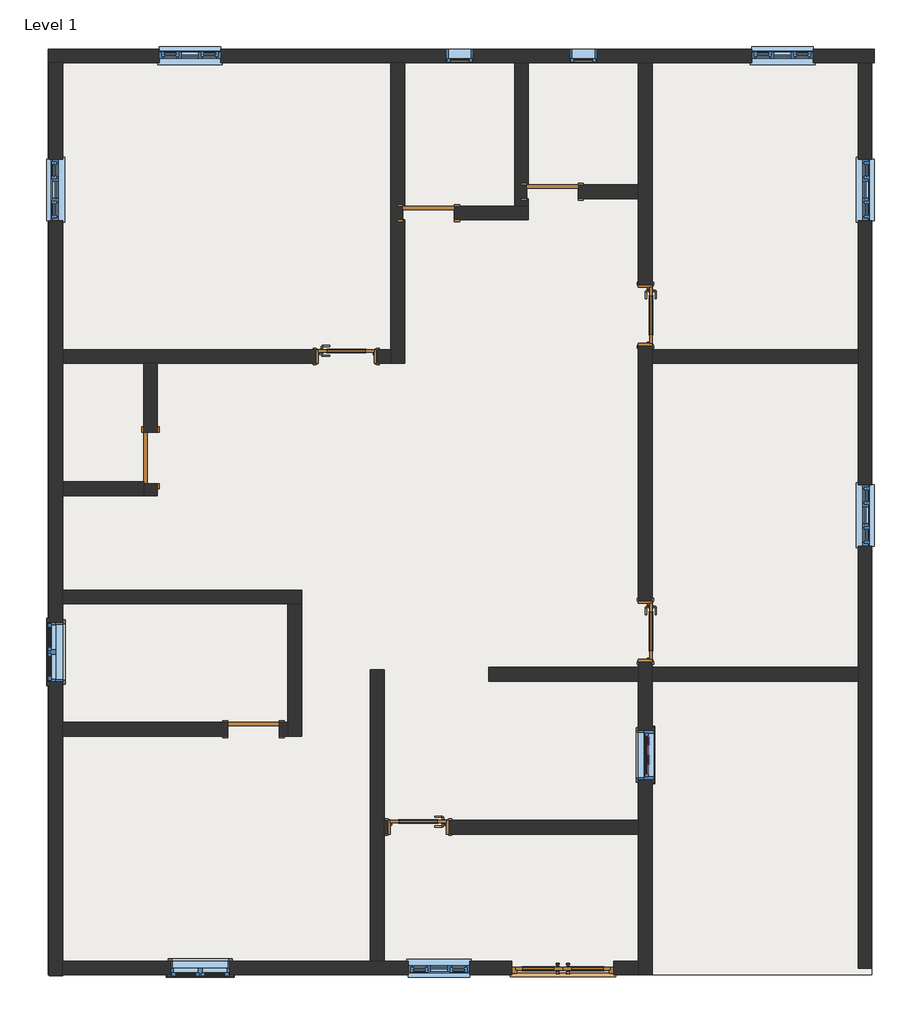
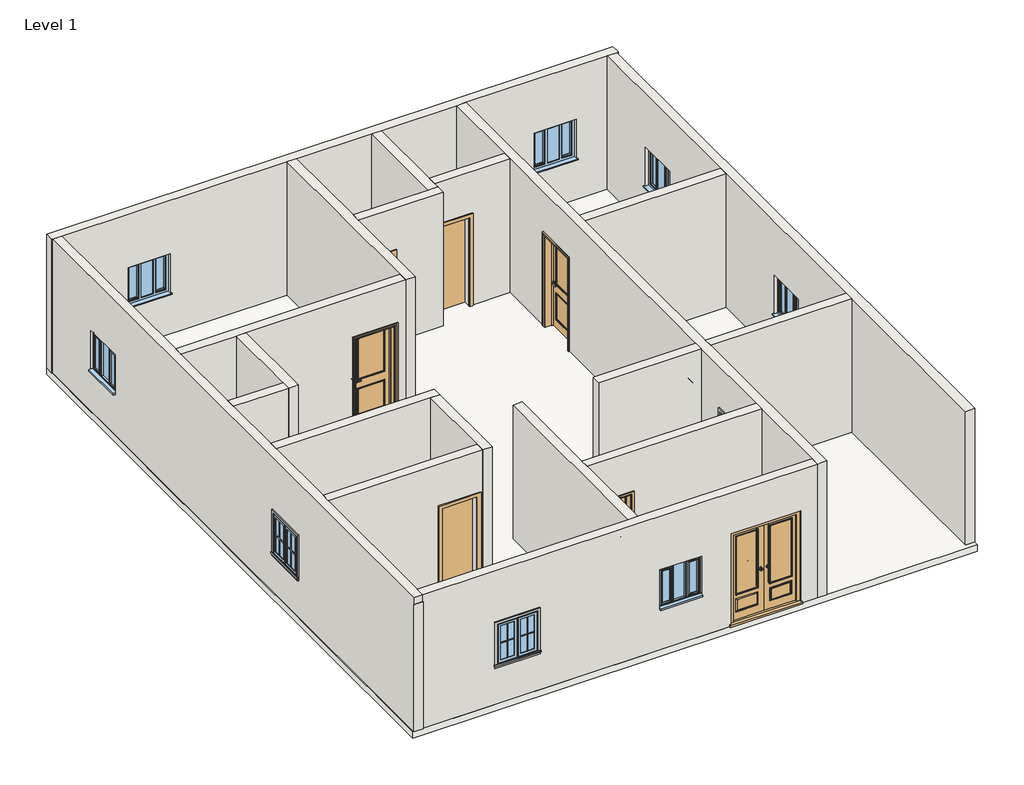
# One storey, incomplete: 19 walls, 12 proxies, 11 windows, 9 doors, 1 slab.
# Revit data of these elements (continued)
# Element 43 (IfcWindow, "Fixed : 16\" x 24\"") (continued)
#   Materials on its faces: "Sash", "Glass"
# Element 44 (IfcWindow, "Window-Casement-Double : 34\" x 36\"")
#   Mark = "1"
#   Window Inset = 0' - 0"
#   Interior Wall Closure = 0' - 2 1/4"
#   Frame Extension = 0' - 0 1/4"
#   Exterior Wall Closure = 0' - 1 1/4"
#   Interior Trim Visibility = yes
#   Exterior Trim Visibility = yes
#   Phase Created = New Construction
#   Materials on its faces: "Wood - Stained", "Glass", "Clad - White"
# Element 45 (IfcWindow, "Window-Casement-Double : 34\" x 36\"")
#   Mark = "2"
#   Window Inset = 0' - 0"
#   Interior Wall Closure = 0' - 2 1/4"
#   Frame Extension = 0' - 0 1/4"
#   Exterior Wall Closure = 0' - 1 1/4"
#   Interior Trim Visibility = yes
#   Exterior Trim Visibility = yes
#   Phase Created = New Construction
#   Materials on its faces: "Wood - Stained", "Glass", "Clad - White"
# Element 46 (IfcWindow, "Window-Double-Hung : 28\" x 46\"")
#   Mark = "11"
#   Window Inset = 0' - 0"
#   Interior Wall Closure = 0' - 1 1/2"
#   Frame Extension = 0' - 1 1/4"
#   Exterior Wall Closure = 0' - 0 1/2"
#   Interior Trim Visibility = yes
#   Indicator Visibility = yes
#   Exterior Trim Visibility = yes
#   Phase Created = New Construction
#   Materials on its faces: "Wood - Stained", "Glass", "Clad - White"
# Element 47 (IfcWindow, "Windows_Tpl_Plain : 910x910mm")
#   Mark = "3"
#   Phase Created = New Construction
#   Materials on its faces: "Window Frame", "Glass"
# Element 48 (IfcWindow, "Windows_Tpl_Plain : 910x910mm")
#   Mark = "6"
#   Phase Created = New Construction
#   Materials on its faces: "Window Frame", "Glass"
# Element 49 (IfcWindow, "Windows_Tpl_Plain : 910x910mm")
#   Mark = "7"
#   Phase Created = New Construction
#   Materials on its faces: "Window Frame", "Glass"
# Element 50 (IfcWindow, "Windows_Tpl_Plain : 910x910mm")
#   Mark = "8"
#   Phase Created = New Construction
#   Materials on its faces: "Window Frame", "Glass"
# Element 51 (IfcWindow, "Windows_Tpl_Plain : 910x910mm")
#   Mark = "4"
#   Phase Created = New Construction
#   Materials on its faces: "Window Frame", "Glass"
# Element 52 (IfcWindow, "Windows_Tpl_Plain : 910x910mm")
#   Mark = "5"
#   Phase Created = New Construction
#   Materials on its faces: "Window Frame", "Glass"
# Materials
#   "Door - Panel": class "Wood", colour RGB 210 159 95, transparency 0, Cost = 0
#   "Door - Glazing": colour RGB 0 0 255, transparency 0.75
#   "Door - Frame/Mullion": class "Wood", colour RGB 212 179 113, transparency 0
#   "Door - Handle": colour RGB 247 247 247, transparency 0
#   "Door - Architrave": class "Wood", colour RGB 154 90 5, transparency 0
#   "Door - Frame": colour RGB 118 70 51, transparency 0, Cost = 0
#   "Glass": class "Glass", colour RGB 0 128 192, transparency 0.75, Description = "Soda Lime Glass", Cost = 0
#   "Sash": class "Wood", colour RGB 224 178 126, transparency 0, Cost = 0
#   "Wood - Stained": class "Wood", colour RGB 224 178 126, transparency 0, Cost = 0
#   "Clad - White": class "Wood", colour RGB 242 242 238, transparency 0, Cost = 0
#   "Window Frame": colour RGB 249 249 249, transparency 0
#   "Default Floor": colour RGB 128 128 128, transparency 0, Cost = 0
#   "Default Wall": colour RGB 128 128 128, transparency 0, Cost = 0
#   "Render Material 255-0-255": colour RGB 255 0 255, transparency 0
